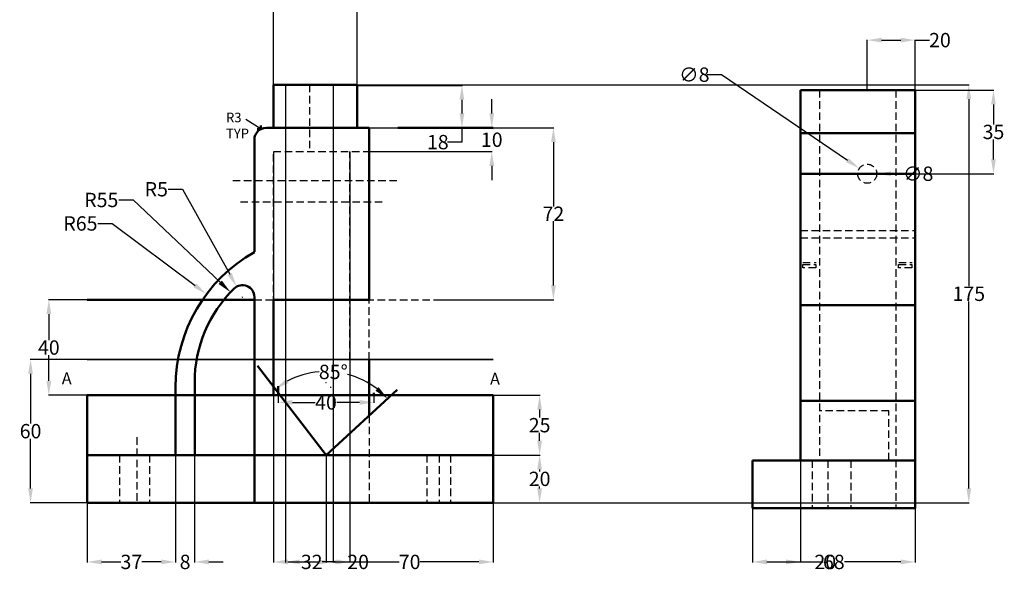
# Model space of a CAD drawing. Units: inches. Extents: x 537 to 975, y 162 to 623.
# Tile 1 of 2: x 563 to 975, y 162 to 393. Entities that reach past the tile are written whole.
import ezdxf

# ---------------------------------------------------------------- set-up
doc = ezdxf.new("R2010")
doc.units = ezdxf.units.IN
doc.header["$LTSCALE"] = 5
doc.header["$MEASUREMENT"] = 0
doc.linetypes.add('HIDDEN2', pattern=[0.1875, 0.125, -0.0625])
doc.linetypes.add('PHANTOM', pattern=[63.5, 31.75, -6.35, 6.35, -6.35, 6.35, -6.35])
for name, color, linetype, lineweight in [('M-DIMS', 2, 'Continuous', 25), ('M-HIDN', 4, 'HIDDEN2', 25), ('M-OUTL', 7, 'Continuous', 50), ('M-SECT', 1, 'PHANTOM', 35), ('M-TEXT', 3, 'Continuous', 25)]:
    doc.layers.add(name, color=color, linetype=linetype, lineweight=lineweight)
doc.styles.get("Standard").update_dxf_attribs({"font": 'arial.ttf'})
doc.dimstyles.get("Standard").update_dxf_attribs({"dimtxt": 6, "dimasz": 6, "dimexe": 0.18, "dimexo": 0.0625, "dimgap": 0.09, "dimtad": 0, "dimtih": 1, "dimtoh": 1, "dimdec": 0, "dimzin": 0, "dimdsep": 46, "dimtxsty": 'Standard', "dimcen": 0.09, "dimadec": 0, "dimazin": 0, "dimtfac": 1, "dimtdec": 0, "dimtofl": 0, "dimtmove": 0, "dimatfit": 3, "dimfxl": 1, "dimtolj": 1, "dimtzin": 0, "dimarcsym": 0})

# ---------------------------------------------------------------- blocks, each defined once
blk = doc.blocks.new('*D15')
at = {"layer": 'Defpoints', "color": 0, "lineweight": 30, "ltscale": 5, "transparency": 16777216}
for p in [(662.25, 248.32), (702.39, 243.97), (720.66, 238.22), (690.92, 210.97), (690.92, 210.97)]:
    blk.add_point(p, dxfattribs=at)
at = {"layer": 'M-DIMS', "color": 0, "lineweight": -2, "ltscale": 5, "transparency": 16777216}
for start, end in [(94.8184, 117.6478), (52.3522, 75.0302)]:
    blk.add_arc((690.92, 210.97), 34.94, start, end, dxfattribs=at)
at = {"layer": 'M-DIMS', "color": 0, "lineweight": 30, "ltscale": 5, "transparency": 16777216}
for points in [[(675.24, 241.07), (674.17, 242.76), (669.65, 238.68)], [(712.93, 239.37), (711.58, 237.89), (716.67, 234.57)]]:
    blk.add_solid(points, dxfattribs=at)
at = {"layer": 'M-DIMS', "color": 0, "ltscale": 5, "transparency": 16777216, "insert": (693.96, 245.77), "char_height": 6, "attachment_point": 5}
blk.add_mtext('\\A1;85°', dxfattribs=at)
blk = doc.blocks.new('*D16')
at = {"layer": 'Defpoints', "color": 0, "lineweight": 30, "ltscale": 5, "transparency": 16777216}
for p in [(670.86, 235.97), (710.92, 235.97), (710.92, 233.01)]:
    blk.add_point(p, dxfattribs=at)
at = {"layer": 'M-DIMS', "color": 0, "lineweight": -2, "ltscale": 5, "transparency": 16777216}
for p, q in [((670.86, 235.9), (670.86, 232.83)), ((710.92, 235.9), (710.92, 232.83)), ((676.86, 233.01), (686.39, 233.01)), ((704.92, 233.01), (695.38, 233.01))]:
    blk.add_line(p, q, dxfattribs=at)
at = {"layer": 'M-DIMS', "color": 0, "lineweight": 30, "ltscale": 5, "transparency": 16777216}
for points in [[(676.86, 234.01), (676.86, 232.01), (670.86, 233.01)], [(704.92, 234.01), (704.92, 232.01), (710.92, 233.01)]]:
    blk.add_solid(points, dxfattribs=at)
at = {"layer": 'M-DIMS', "color": 0, "ltscale": 5, "transparency": 16777216, "insert": (690.89, 233.01), "char_height": 6, "attachment_point": 5}
blk.add_mtext('\\A1;40', dxfattribs=at)
blk = doc.blocks.new('*D17')
at = {"layer": 'Defpoints', "color": 0, "lineweight": 30, "ltscale": 5, "transparency": 16777216}
for p in [(760.92, 210.97), (780.32, 210.97), (758.37, 191.01)]:
    blk.add_point(p, dxfattribs=at)
at = {"layer": 'M-DIMS', "color": 0, "lineweight": -2, "ltscale": 5, "transparency": 16777216}
for p, q in [((760.98, 210.97), (780.5, 210.97)), ((780.32, 204.97), (780.32, 204.14)), ((780.32, 197.01), (780.32, 197.84)), ((758.44, 191.01), (780.5, 191.01))]:
    blk.add_line(p, q, dxfattribs=at)
at = {"layer": 'M-DIMS', "color": 0, "lineweight": 30, "ltscale": 5, "transparency": 16777216}
for points in [[(779.32, 204.97), (781.32, 204.97), (780.32, 210.97)], [(779.32, 197.01), (781.32, 197.01), (780.32, 191.01)]]:
    blk.add_solid(points, dxfattribs=at)
at = {"layer": 'M-DIMS', "color": 0, "ltscale": 5, "transparency": 16777216, "insert": (780.32, 200.99), "char_height": 6, "attachment_point": 5}
blk.add_mtext('\\A1;20', dxfattribs=at)
blk = doc.blocks.new('*D18')
at = {"layer": 'Defpoints', "color": 0, "lineweight": 30, "ltscale": 5, "transparency": 16777216}
for p in [(760.92, 235.97), (780.32, 235.97), (760.92, 210.97)]:
    blk.add_point(p, dxfattribs=at)
at = {"layer": 'M-DIMS', "color": 0, "lineweight": -2, "ltscale": 5, "transparency": 16777216}
for p, q in [((760.98, 235.97), (780.5, 235.97)), ((780.32, 229.97), (780.32, 226.62)), ((780.32, 216.97), (780.32, 220.31)), ((760.98, 210.97), (780.5, 210.97))]:
    blk.add_line(p, q, dxfattribs=at)
at = {"layer": 'M-DIMS', "color": 0, "lineweight": 30, "ltscale": 5, "transparency": 16777216}
for points in [[(779.32, 229.97), (781.32, 229.97), (780.32, 235.97)], [(779.32, 216.97), (781.32, 216.97), (780.32, 210.97)]]:
    blk.add_solid(points, dxfattribs=at)
at = {"layer": 'M-DIMS', "color": 0, "ltscale": 5, "transparency": 16777216, "insert": (780.32, 223.47), "char_height": 6, "attachment_point": 5}
blk.add_mtext('\\A1;25', dxfattribs=at)
blk = doc.blocks.new('*D19')
at = {"layer": 'Defpoints', "color": 0, "lineweight": 30, "ltscale": 5, "transparency": 16777216}
for p in [(567.22, 250.97), (590.92, 250.97), (590.92, 190.97)]:
    blk.add_point(p, dxfattribs=at)
at = {"layer": 'M-DIMS', "color": 0, "lineweight": -2, "ltscale": 5, "transparency": 16777216}
for p, q in [((590.85, 250.97), (567.04, 250.97)), ((567.22, 244.97), (567.22, 224.12)), ((567.22, 196.97), (567.22, 217.81)), ((590.85, 190.97), (567.04, 190.97))]:
    blk.add_line(p, q, dxfattribs=at)
at = {"layer": 'M-DIMS', "color": 0, "lineweight": 30, "ltscale": 5, "transparency": 16777216}
for points in [[(566.22, 244.97), (568.22, 244.97), (567.22, 250.97)], [(566.22, 196.97), (568.22, 196.97), (567.22, 190.97)]]:
    blk.add_solid(points, dxfattribs=at)
at = {"layer": 'M-DIMS', "color": 0, "ltscale": 5, "transparency": 16777216, "insert": (567.22, 220.97), "char_height": 6, "attachment_point": 5}
blk.add_mtext('\\A1;60', dxfattribs=at)
blk = doc.blocks.new('*D20')
at = {"layer": 'Defpoints', "color": 0, "lineweight": 30, "ltscale": 5, "transparency": 16777216}
for p in [(574.87, 275.97), (590.92, 275.97), (590.92, 235.97)]:
    blk.add_point(p, dxfattribs=at)
at = {"layer": 'M-DIMS', "color": 0, "lineweight": -2, "ltscale": 5, "transparency": 16777216}
for p, q in [((590.85, 275.97), (574.69, 275.97)), ((574.87, 269.97), (574.87, 259.12)), ((574.87, 241.97), (574.87, 252.81)), ((590.85, 235.97), (574.69, 235.97))]:
    blk.add_line(p, q, dxfattribs=at)
at = {"layer": 'M-DIMS', "color": 0, "lineweight": 30, "ltscale": 5, "transparency": 16777216}
for points in [[(573.87, 269.97), (575.87, 269.97), (574.87, 275.97)], [(573.87, 241.97), (575.87, 241.97), (574.87, 235.97)]]:
    blk.add_solid(points, dxfattribs=at)
at = {"layer": 'M-DIMS', "color": 0, "ltscale": 5, "transparency": 16777216, "insert": (574.87, 255.97), "char_height": 6, "attachment_point": 5}
blk.add_mtext('\\A1;40', dxfattribs=at)
blk = doc.blocks.new('*D21')
at = {"layer": 'Defpoints', "color": 0, "lineweight": 30, "ltscale": 5, "transparency": 16777216}
for p in [(737.44, 347.97), (786.09, 347.97), (737.44, 275.97)]:
    blk.add_point(p, dxfattribs=at)
at = {"layer": 'M-DIMS', "color": 0, "lineweight": -2, "ltscale": 5, "transparency": 16777216}
for p, q in [((737.5, 347.97), (786.27, 347.97)), ((786.09, 341.97), (786.09, 315.07)), ((786.09, 281.97), (786.09, 308.87)), ((737.5, 275.97), (786.27, 275.97))]:
    blk.add_line(p, q, dxfattribs=at)
at = {"layer": 'M-DIMS', "color": 0, "lineweight": 30, "ltscale": 5, "transparency": 16777216}
for points in [[(785.09, 341.97), (787.09, 341.97), (786.09, 347.97)], [(785.09, 281.97), (787.09, 281.97), (786.09, 275.97)]]:
    blk.add_solid(points, dxfattribs=at)
at = {"layer": 'M-DIMS', "color": 0, "ltscale": 5, "transparency": 16777216, "insert": (786.09, 311.97), "char_height": 6, "attachment_point": 5}
blk.add_mtext('\\A1;72', dxfattribs=at)
blk = doc.blocks.new('*D22')
at = {"layer": 'Defpoints', "color": 0, "lineweight": 30, "ltscale": 5, "transparency": 16777216}
for p in [(708.92, 347.97), (760.28, 347.97), (708.92, 337.97)]:
    blk.add_point(p, dxfattribs=at)
at = {"layer": 'M-DIMS', "color": 0, "lineweight": -2, "ltscale": 5, "transparency": 16777216}
for p, q in [((760.28, 353.97), (760.28, 359.97)), ((708.98, 347.97), (760.46, 347.97)), ((708.98, 337.97), (760.46, 337.97)), ((760.28, 331.97), (760.28, 325.97))]:
    blk.add_line(p, q, dxfattribs=at)
at = {"layer": 'M-DIMS', "color": 0, "lineweight": 30, "ltscale": 5, "transparency": 16777216}
for points in [[(759.28, 353.97), (761.28, 353.97), (760.28, 347.97)], [(759.28, 331.97), (761.28, 331.97), (760.28, 337.97)]]:
    blk.add_solid(points, dxfattribs=at)
at = {"layer": 'M-DIMS', "color": 0, "ltscale": 5, "transparency": 16777216, "insert": (760.28, 342.97), "char_height": 6, "attachment_point": 5}
blk.add_mtext('\\A1;10', dxfattribs=at)
blk = doc.blocks.new('*D23')
at = {"layer": 'Defpoints', "color": 0, "lineweight": 30, "ltscale": 5, "transparency": 16777216}
for p in [(703.92, 365.68), (703.92, 347.97), (747.8, 347.97)]:
    blk.add_point(p, dxfattribs=at)
at = {"layer": 'M-DIMS', "color": 0, "lineweight": -2, "ltscale": 5, "transparency": 16777216}
for p, q in [((703.98, 365.68), (747.98, 365.68)), ((747.8, 359.68), (747.8, 353.97)), ((703.98, 347.97), (747.98, 347.97)), ((747.8, 347.97), (747.8, 341.97)), ((747.8, 341.97), (741.8, 341.97))]:
    blk.add_line(p, q, dxfattribs=at)
at = {"layer": 'M-DIMS', "color": 0, "lineweight": 30, "ltscale": 5, "transparency": 16777216}
for points in [[(746.8, 359.68), (748.8, 359.68), (747.8, 365.68)], [(746.8, 353.97), (748.8, 353.97), (747.8, 347.97)]]:
    blk.add_solid(points, dxfattribs=at)
at = {"layer": 'M-DIMS', "color": 0, "ltscale": 5, "transparency": 16777216, "insert": (737.69, 341.97), "char_height": 6, "attachment_point": 5}
blk.add_mtext('\\A1;18', dxfattribs=at)
blk = doc.blocks.new('*D24')
at = {"layer": 'Defpoints', "color": 0, "lineweight": 30, "ltscale": 5, "transparency": 16777216}
for p in [(653.49, 281.47), (655.92, 277.1)]:
    blk.add_point(p, dxfattribs=at)
at = {"layer": 'M-DIMS', "color": 0, "lineweight": -2, "ltscale": 5, "transparency": 16777216}
for p, q in [((624.82, 322.24), (630.82, 322.24)), ((630.82, 322.24), (650.57, 286.71)), ((655.83, 277.1), (656.01, 277.1)), ((655.92, 277.01), (655.92, 277.19))]:
    blk.add_line(p, q, dxfattribs=at)
at = {"layer": 'M-DIMS', "color": 0, "lineweight": 30, "ltscale": 5, "transparency": 16777216}
blk.add_solid([(651.44, 287.2), (649.7, 286.23), (653.49, 281.47)], dxfattribs=at)
at = {"layer": 'M-DIMS', "color": 0, "ltscale": 5, "transparency": 16777216, "insert": (619.86, 322.24), "char_height": 6, "attachment_point": 5}
blk.add_mtext('\\A1;R5', dxfattribs=at)
blk = doc.blocks.new('*D25')
at = {"layer": 'Defpoints', "color": 0, "lineweight": 30, "ltscale": 5, "transparency": 16777216}
for p in [(640.88, 278.34), (692.92, 239.39)]:
    blk.add_point(p, dxfattribs=at)
at = {"layer": 'M-DIMS', "color": 0, "lineweight": -2, "ltscale": 5, "transparency": 16777216}
for p, q in [((595.38, 307.91), (601.38, 307.91)), ((601.38, 307.91), (636.07, 281.94)), ((692.83, 239.39), (693.01, 239.39)), ((692.92, 239.3), (692.92, 239.48))]:
    blk.add_line(p, q, dxfattribs=at)
at = {"layer": 'M-DIMS', "color": 0, "lineweight": 30, "ltscale": 5, "transparency": 16777216}
blk.add_solid([(636.67, 282.74), (635.47, 281.14), (640.88, 278.34)], dxfattribs=at)
at = {"layer": 'M-DIMS', "color": 0, "ltscale": 5, "transparency": 16777216, "insert": (588.1, 307.91), "char_height": 6, "attachment_point": 5}
blk.add_mtext('\\A1;R65', dxfattribs=at)
blk = doc.blocks.new('*D26')
at = {"layer": 'Defpoints', "color": 0, "lineweight": 30, "ltscale": 5, "transparency": 16777216}
for p in [(650.94, 279.17), (690.92, 241.39)]:
    blk.add_point(p, dxfattribs=at)
at = {"layer": 'M-DIMS', "color": 0, "lineweight": -2, "ltscale": 5, "transparency": 16777216}
for p, q in [((604.11, 317.75), (610.11, 317.75)), ((610.11, 317.75), (646.58, 283.29)), ((690.83, 241.39), (691.01, 241.39)), ((690.92, 241.3), (690.92, 241.48))]:
    blk.add_line(p, q, dxfattribs=at)
at = {"layer": 'M-DIMS', "color": 0, "lineweight": 30, "ltscale": 5, "transparency": 16777216}
blk.add_solid([(647.27, 284.02), (645.89, 282.56), (650.94, 279.17)], dxfattribs=at)
at = {"layer": 'M-DIMS', "color": 0, "ltscale": 5, "transparency": 16777216, "insert": (596.83, 317.75), "char_height": 6, "attachment_point": 5}
blk.add_mtext('\\A1;R55', dxfattribs=at)
blk = doc.blocks.new('*D27')
at = {"layer": 'Defpoints', "color": 0, "lineweight": 30, "ltscale": 5, "transparency": 16777216}
for p in [(914.16, 330.98), (920.78, 326.49)]:
    blk.add_point(p, dxfattribs=at)
at = {"layer": 'M-DIMS', "color": 0, "lineweight": -2, "ltscale": 5, "transparency": 16777216}
for p, q in [((850.41, 370.21), (856.41, 370.21)), ((856.41, 370.21), (909.2, 334.35)), ((917.38, 328.73), (917.56, 328.73)), ((917.47, 328.64), (917.47, 328.82))]:
    blk.add_line(p, q, dxfattribs=at)
at = {"layer": 'M-DIMS', "color": 0, "lineweight": 30, "ltscale": 5, "transparency": 16777216}
blk.add_solid([(909.76, 335.18), (908.63, 333.53), (914.16, 330.98)], dxfattribs=at)
at = {"layer": 'M-DIMS', "color": 0, "ltscale": 5, "transparency": 16777216, "insert": (845.08, 370.21), "char_height": 6, "attachment_point": 5}
blk.add_mtext('\\A1;∅8', dxfattribs=at)
blk = doc.blocks.new('*D28')
at = {"layer": 'Defpoints', "color": 0, "lineweight": 30, "ltscale": 5, "transparency": 16777216}
for p in [(937.47, 384.67), (917.47, 363.73), (937.47, 363.73)]:
    blk.add_point(p, dxfattribs=at)
at = {"layer": 'M-DIMS', "color": 0, "lineweight": -2, "ltscale": 5, "transparency": 16777216}
for p, q in [((917.47, 363.8), (917.47, 384.85)), ((923.47, 384.67), (931.47, 384.67)), ((937.47, 363.8), (937.47, 384.85)), ((937.47, 384.67), (943.47, 384.67))]:
    blk.add_line(p, q, dxfattribs=at)
at = {"layer": 'M-DIMS', "color": 0, "lineweight": 30, "ltscale": 5, "transparency": 16777216}
for points in [[(923.47, 385.67), (923.47, 383.67), (917.47, 384.67)], [(931.47, 385.67), (931.47, 383.67), (937.47, 384.67)]]:
    blk.add_solid(points, dxfattribs=at)
at = {"layer": 'M-DIMS', "color": 0, "ltscale": 5, "transparency": 16777216, "insert": (947.9, 384.67), "char_height": 6, "attachment_point": 5}
blk.add_mtext('\\A1;20', dxfattribs=at)
blk = doc.blocks.new('*D29')
at = {"layer": 'Defpoints', "color": 0, "lineweight": 30, "ltscale": 5, "transparency": 16777216}
for p in [(937.47, 363.73), (937.47, 328.73), (970.3, 328.73)]:
    blk.add_point(p, dxfattribs=at)
at = {"layer": 'M-DIMS', "color": 0, "lineweight": -2, "ltscale": 5, "transparency": 16777216}
for p, q in [((937.53, 363.73), (970.48, 363.73)), ((970.3, 357.73), (970.3, 349.39)), ((970.3, 334.73), (970.3, 343.08)), ((937.53, 328.73), (970.48, 328.73))]:
    blk.add_line(p, q, dxfattribs=at)
at = {"layer": 'M-DIMS', "color": 0, "lineweight": 30, "ltscale": 5, "transparency": 16777216}
for points in [[(969.3, 357.73), (971.3, 357.73), (970.3, 363.73)], [(969.3, 334.73), (971.3, 334.73), (970.3, 328.73)]]:
    blk.add_solid(points, dxfattribs=at)
at = {"layer": 'M-DIMS', "color": 0, "ltscale": 5, "transparency": 16777216, "insert": (970.3, 346.23), "char_height": 6, "attachment_point": 5}
blk.add_mtext('\\A1;35', dxfattribs=at)
blk = doc.blocks.new('*D30')
at = {"layer": 'Defpoints', "color": 0, "lineweight": 30, "ltscale": 5, "transparency": 16777216}
for p in [(627.92, 239.39), (590.92, 190.97), (627.92, 166.23)]:
    blk.add_point(p, dxfattribs=at)
at = {"layer": 'M-DIMS', "color": 0, "lineweight": -2, "ltscale": 5, "transparency": 16777216}
for p, q in [((627.92, 239.33), (627.92, 166.05)), ((590.92, 190.9), (590.92, 166.05)), ((596.92, 166.23), (605.03, 166.23)), ((621.92, 166.23), (613.8, 166.23))]:
    blk.add_line(p, q, dxfattribs=at)
at = {"layer": 'M-DIMS', "color": 0, "lineweight": 30, "ltscale": 5, "transparency": 16777216}
for points in [[(596.92, 167.23), (596.92, 165.23), (590.92, 166.23)], [(621.92, 167.23), (621.92, 165.23), (627.92, 166.23)]]:
    blk.add_solid(points, dxfattribs=at)
at = {"layer": 'M-DIMS', "color": 0, "ltscale": 5, "transparency": 16777216, "insert": (609.42, 166.23), "char_height": 6, "attachment_point": 5}
blk.add_mtext('\\A1;37', dxfattribs=at)
blk = doc.blocks.new('*D31')
at = {"layer": 'Defpoints', "color": 0, "lineweight": 30, "ltscale": 5, "transparency": 16777216}
for p in [(627.91595, 210.967485), (635.91595, 210.967485), (635.91595, 166.233266)]:
    blk.add_point(p, dxfattribs=at)
at = {"layer": 'M-DIMS', "color": 0, "lineweight": -2, "ltscale": 5, "transparency": 16777216}
for p, q in [((627.91595, 210.904985), (627.91595, 166.053266)), ((635.91595, 210.904985), (635.91595, 166.053266)), ((621.91595, 166.233266), (615.91595, 166.233266)), ((641.91595, 166.233266), (647.91595, 166.233266))]:
    blk.add_line(p, q, dxfattribs=at)
at = {"layer": 'M-DIMS', "color": 0, "lineweight": 30, "ltscale": 5, "transparency": 16777216}
for points in [[(621.91595, 167.233266), (621.91595, 165.233266), (627.91595, 166.233266)], [(641.91595, 167.233266), (641.91595, 165.233266), (635.91595, 166.233266)]]:
    blk.add_solid(points, dxfattribs=at)
at = {"layer": 'M-DIMS', "color": 0, "ltscale": 5, "transparency": 16777216, "insert": (631.91595, 166.233266), "char_height": 6, "attachment_point": 5}
blk.add_mtext('\\A1;8', dxfattribs=at)
blk = doc.blocks.new('*D32')
at = {"layer": 'Defpoints', "color": 0, "lineweight": 30, "ltscale": 5, "transparency": 16777216}
for p in [(690.92, 210.97), (760.92, 190.97), (690.92, 166.23)]:
    blk.add_point(p, dxfattribs=at)
at = {"layer": 'M-DIMS', "color": 0, "lineweight": -2, "ltscale": 5, "transparency": 16777216}
for p, q in [((690.92, 210.9), (690.92, 166.05)), ((760.92, 190.9), (760.92, 166.05)), ((696.92, 166.23), (721.56, 166.23)), ((754.92, 166.23), (730.27, 166.23))]:
    blk.add_line(p, q, dxfattribs=at)
at = {"layer": 'M-DIMS', "color": 0, "lineweight": 30, "ltscale": 5, "transparency": 16777216}
for points in [[(696.92, 167.23), (696.92, 165.23), (690.92, 166.23)], [(754.92, 167.23), (754.92, 165.23), (760.92, 166.23)]]:
    blk.add_solid(points, dxfattribs=at)
at = {"layer": 'M-DIMS', "color": 0, "ltscale": 5, "transparency": 16777216, "insert": (725.92, 166.23), "char_height": 6, "attachment_point": 5}
blk.add_mtext('\\A1;70', dxfattribs=at)
blk = doc.blocks.new('*D33')
at = {"layer": 'Defpoints', "color": 0, "lineweight": 30, "ltscale": 5, "transparency": 16777216}
for p in [(703.92, 619.5), (668.92, 365.97), (703.92, 365.97)]:
    blk.add_point(p, dxfattribs=at)
at = {"layer": 'M-DIMS', "color": 0, "lineweight": -2, "ltscale": 5, "transparency": 16777216}
for p, q in [((668.92, 366.03), (668.92, 619.68)), ((674.92, 619.5), (682.01, 619.5)), ((697.92, 619.5), (690.82, 619.5)), ((703.92, 366.03), (703.92, 619.68))]:
    blk.add_line(p, q, dxfattribs=at)
at = {"layer": 'M-DIMS', "color": 0, "lineweight": 30, "ltscale": 5, "transparency": 16777216}
for points in [[(674.92, 620.5), (674.92, 618.5), (668.92, 619.5)], [(697.92, 620.5), (697.92, 618.5), (703.92, 619.5)]]:
    blk.add_solid(points, dxfattribs=at)
at = {"layer": 'M-DIMS', "color": 0, "ltscale": 5, "transparency": 16777216, "insert": (686.42, 619.5), "char_height": 6, "attachment_point": 5}
blk.add_mtext('\\A1;35', dxfattribs=at)
blk = doc.blocks.new('*D34')
at = {"layer": 'Defpoints', "color": 0, "lineweight": 30, "ltscale": 5, "transparency": 16777216}
for p in [(668.92, 337.97), (700.92, 337.97), (700.92, 166.23)]:
    blk.add_point(p, dxfattribs=at)
at = {"layer": 'M-DIMS', "color": 0, "lineweight": -2, "ltscale": 5, "transparency": 16777216}
for p, q in [((668.92, 337.9), (668.92, 166.05)), ((700.92, 337.9), (700.92, 166.05)), ((674.92, 166.23), (680.56, 166.23)), ((694.92, 166.23), (689.27, 166.23))]:
    blk.add_line(p, q, dxfattribs=at)
at = {"layer": 'M-DIMS', "color": 0, "lineweight": 30, "ltscale": 5, "transparency": 16777216}
for points in [[(674.92, 167.23), (674.92, 165.23), (668.92, 166.23)], [(694.92, 167.23), (694.92, 165.23), (700.92, 166.23)]]:
    blk.add_solid(points, dxfattribs=at)
at = {"layer": 'M-DIMS', "color": 0, "ltscale": 5, "transparency": 16777216, "insert": (684.92, 166.23), "char_height": 6, "attachment_point": 5}
blk.add_mtext('\\A1;32', dxfattribs=at)
blk = doc.blocks.new('*D35')
at = {"layer": 'Defpoints', "color": 0, "lineweight": 30, "ltscale": 5, "transparency": 16777216}
for p in [(673.92, 365.97), (693.92, 365.97), (693.92, 166.23)]:
    blk.add_point(p, dxfattribs=at)
at = {"layer": 'M-DIMS', "color": 0, "lineweight": -2, "ltscale": 5, "transparency": 16777216}
for p, q in [((673.92, 365.9), (673.92, 166.05)), ((693.92, 365.9), (693.92, 166.05)), ((679.92, 166.23), (687.92, 166.23)), ((693.92, 166.23), (699.92, 166.23))]:
    blk.add_line(p, q, dxfattribs=at)
at = {"layer": 'M-DIMS', "color": 0, "lineweight": 30, "ltscale": 5, "transparency": 16777216}
for points in [[(679.92, 167.23), (679.92, 165.23), (673.92, 166.23)], [(687.92, 167.23), (687.92, 165.23), (693.92, 166.23)]]:
    blk.add_solid(points, dxfattribs=at)
at = {"layer": 'M-DIMS', "color": 0, "ltscale": 5, "transparency": 16777216, "insert": (704.34, 166.23), "char_height": 6, "attachment_point": 5}
blk.add_mtext('\\A1;20', dxfattribs=at)
blk = doc.blocks.new('*D36')
at = {"layer": 'Defpoints', "color": 0, "lineweight": 30, "ltscale": 5, "transparency": 16777216}
for p in [(703.92, 365.97), (959.97, 365.97), (760.92, 190.97)]:
    blk.add_point(p, dxfattribs=at)
at = {"layer": 'M-DIMS', "color": 0, "lineweight": -2, "ltscale": 5, "transparency": 16777216}
for p, q in [((703.98, 365.97), (960.15, 365.97)), ((959.97, 359.97), (959.97, 281.62)), ((959.97, 196.97), (959.97, 275.31)), ((760.98, 190.97), (960.15, 190.97))]:
    blk.add_line(p, q, dxfattribs=at)
at = {"layer": 'M-DIMS', "color": 0, "lineweight": 30, "ltscale": 5, "transparency": 16777216}
for points in [[(958.97, 359.97), (960.97, 359.97), (959.97, 365.97)], [(958.97, 196.97), (960.97, 196.97), (959.97, 190.97)]]:
    blk.add_solid(points, dxfattribs=at)
at = {"layer": 'M-DIMS', "color": 0, "ltscale": 5, "transparency": 16777216, "insert": (959.97, 278.47), "char_height": 6, "attachment_point": 5}
blk.add_mtext('\\A1;175', dxfattribs=at)
blk = doc.blocks.new('*D37')
at = {"layer": 'Defpoints', "color": 0, "lineweight": 30, "ltscale": 5, "transparency": 16777216}
for p in [(869.47, 188.73), (937.47, 188.73), (937.47, 166.23)]:
    blk.add_point(p, dxfattribs=at)
at = {"layer": 'M-DIMS', "color": 0, "lineweight": -2, "ltscale": 5, "transparency": 16777216}
for p, q in [((869.47, 188.67), (869.47, 166.05)), ((937.47, 188.67), (937.47, 166.05)), ((875.47, 166.23), (899.06, 166.23)), ((931.47, 166.23), (907.88, 166.23))]:
    blk.add_line(p, q, dxfattribs=at)
at = {"layer": 'M-DIMS', "color": 0, "lineweight": 30, "ltscale": 5, "transparency": 16777216}
for points in [[(875.47, 167.23), (875.47, 165.23), (869.47, 166.23)], [(931.47, 167.23), (931.47, 165.23), (937.47, 166.23)]]:
    blk.add_solid(points, dxfattribs=at)
at = {"layer": 'M-DIMS', "color": 0, "ltscale": 5, "transparency": 16777216, "insert": (903.47, 166.23), "char_height": 6, "attachment_point": 5}
blk.add_mtext('\\A1;68', dxfattribs=at)
blk = doc.blocks.new('*D38')
at = {"layer": 'Defpoints', "color": 0, "lineweight": 30, "ltscale": 5, "transparency": 16777216}
for p in [(869.47, 208.73), (889.47, 208.73), (889.47, 166.23)]:
    blk.add_point(p, dxfattribs=at)
at = {"layer": 'M-DIMS', "color": 0, "lineweight": -2, "ltscale": 5, "transparency": 16777216}
for p, q in [((869.47, 208.67), (869.47, 166.05)), ((889.47, 208.67), (889.47, 166.05)), ((875.47, 166.23), (883.47, 166.23)), ((889.47, 166.23), (895.47, 166.23))]:
    blk.add_line(p, q, dxfattribs=at)
at = {"layer": 'M-DIMS', "color": 0, "lineweight": 30, "ltscale": 5, "transparency": 16777216}
for points in [[(875.47, 167.23), (875.47, 165.23), (869.47, 166.23)], [(883.47, 167.23), (883.47, 165.23), (889.47, 166.23)]]:
    blk.add_solid(points, dxfattribs=at)
at = {"layer": 'M-DIMS', "color": 0, "ltscale": 5, "transparency": 16777216, "insert": (899.9, 166.23), "char_height": 6, "attachment_point": 5}
blk.add_mtext('\\A1;20', dxfattribs=at)
blk = doc.blocks.new('*D41')
at = {"layer": 'Defpoints', "color": 0, "lineweight": 30, "ltscale": 5, "transparency": 16777216}
for p in [(913.47, 328.73), (921.47, 328.73)]:
    blk.add_point(p, dxfattribs=at)
at = {"layer": 'M-DIMS', "color": 0, "lineweight": -2, "ltscale": 5, "transparency": 16777216}
for p, q in [((917.38, 328.73), (917.56, 328.73)), ((917.47, 328.64), (917.47, 328.82)), ((933.47, 328.73), (927.47, 328.73))]:
    blk.add_line(p, q, dxfattribs=at)
at = {"layer": 'M-DIMS', "color": 0, "lineweight": 30, "ltscale": 5, "transparency": 16777216}
blk.add_solid([(927.47, 329.73), (927.47, 327.73), (921.47, 328.73)], dxfattribs=at)
at = {"layer": 'M-DIMS', "color": 0, "ltscale": 5, "transparency": 16777216, "insert": (938.79, 328.73), "char_height": 6, "attachment_point": 5}
blk.add_mtext('\\A1;∅8', dxfattribs=at)

msp = doc.modelspace()

# ---------------------------------------------------------------- linework, layer by layer
at = {"layer": 'M-DIMS', "ltscale": 5}
msp.add_line((663.71, 347.45), (657.28, 351.44), dxfattribs=at)
at = {"layer": 'M-HIDN', "ltscale": 5}
for p, q in [((668.92, 347.97), (668.92, 365.97)), ((673.92, 365.97), (673.92, 337.97)), ((683.92, 365.97), (683.92, 337.97)), ((693.92, 365.97), (693.92, 337.97)), ((703.92, 365.97), (703.92, 347.97)), ((897.47, 363.73), (897.47, 208.73)), ((929.47, 363.73), (929.47, 188.73)), ((660.92, 295.97), (660.92, 342.97)), ((668.92, 291.6), (668.92, 337.97)), ((668.92, 337.97), (708.92, 337.97)), ((700.92, 250.97), (700.92, 337.97)), ((708.92, 250.97), (708.92, 337.97)), ((651.86, 325.94), (721.6, 325.94)), ((655.1, 316.99), (714.93, 316.99)), ((889.47, 304.92), (937.47, 304.92)), ((889.47, 301.92), (937.47, 301.92)), ((668.92, 250.97), (668.92, 291.6)), ((890.51, 291.55), (896.06, 291.55)), ((930.66, 291.55), (936.21, 291.55)), ((660.92, 275.97), (783.9, 275.97)), ((700.92, 250.97), (700.92, 190.97)), ((668.92, 235.97), (668.92, 190.97)), ((708.92, 227.46), (708.92, 190.97)), ((926.51, 229.45), (897.47, 229.45)), ((926.51, 208.73), (926.51, 229.45)), ((611.66, 218.4), (611.66, 190.97)), ((604.4, 210.97), (604.4, 190.97)), ((617.04, 210.97), (617.04, 190.97)), ((733.17, 210.97), (733.17, 190.97)), ((738.3, 210.97), (738.3, 190.97)), ((742.99, 210.97), (742.99, 190.97)), ((894.41, 208.73), (894.41, 188.73)), ((901.02, 208.73), (901.02, 188.73)), ((910.53, 208.73), (910.53, 188.73))]:
    msp.add_line(p, q, dxfattribs=at)
for points in [[(890.45, 290.78), (896.01, 290.78), (896.01, 289.4), (890.45, 289.4)], [(930.6, 290.78), (936.15, 290.78), (936.15, 289.4), (930.6, 289.4)]]:
    msp.add_lwpolyline(points, close=True, dxfattribs=at)
msp.add_circle((917.47, 328.73), 4, dxfattribs=at)
at = {"layer": 'M-OUTL', "ltscale": 5}
for p, q in [((668.92, 365.97), (703.92, 365.97)), ((703.92, 365.97), (668.92, 365.97)), ((668.92, 347.97), (668.92, 365.97)), ((668.92, 365.97), (703.92, 365.97)), ((703.92, 365.97), (703.92, 347.97)), ((889.47, 363.73), (937.47, 363.73)), ((889.47, 363.73), (889.47, 208.73)), ((937.47, 363.73), (937.47, 188.73)), ((663.71, 347.45), (662.07, 347.37)), ((663.71, 347.45), (663.64, 348.88)), ((665.92, 347.97), (708.92, 347.97)), ((665.92, 347.97), (668.92, 347.97)), ((703.92, 347.97), (708.92, 347.97)), ((708.92, 347.97), (708.92, 275.97)), ((720.92, 347.97), (760.92, 347.97)), ((660.92, 295.97), (660.92, 342.97)), ((889.47, 345.73), (937.47, 345.73)), ((889.47, 328.73), (937.47, 328.73)), ((660.92, 277.1), (660.92, 190.97)), ((590.92, 275.97), (660.92, 275.97)), ((668.92, 235.97), (668.92, 275.97)), ((668.92, 275.97), (708.92, 275.97)), ((889.47, 273.73), (937.47, 273.73)), ((690.92, 210.97), (662.25, 248.32)), ((668.92, 250.97), (668.92, 235.97)), ((708.92, 250.97), (708.92, 227.46)), ((627.92, 239.39), (627.92, 210.97)), ((635.92, 241.39), (635.92, 210.97)), ((670.92, 235.97), (670.86, 239.77)), ((590.92, 235.97), (760.92, 235.97)), ((590.92, 190.97), (590.92, 235.97)), ((710.92, 235.97), (670.92, 235.97)), ((700.92, 235.97), (680.92, 235.97)), ((690.92, 210.97), (720.66, 238.22)), ((690.92, 235.97), (710.92, 235.97)), ((710.92, 235.97), (710.92, 237.03)), ((760.92, 190.97), (760.92, 235.97)), ((889.47, 233.73), (937.47, 233.73)), ((590.92, 210.97), (760.92, 210.97)), ((720.92, 210.97), (660.92, 210.97)), ((869.47, 208.73), (937.47, 208.73)), ((869.47, 208.73), (869.47, 188.73)), ((590.92, 190.97), (760.92, 190.97)), ((869.47, 188.73), (937.47, 188.73))]:
    msp.add_line(p, q, dxfattribs=at)
for centre, radius, start, end in [((665.92, 342.97), 5, 90, 180), ((692.92, 239.39), 65, 119.4924, 180), ((690.92, 241.39), 55, 134.427, 180), ((655.92, 277.1), 5, 0, 134.427)]:
    msp.add_arc(centre, radius, start, end, dxfattribs=at)
at = {"layer": 'M-SECT', "ltscale": 5}
msp.add_line((590.92, 250.97), (760.92, 250.97), dxfattribs=at)

# ---------------------------------------------------------------- texts
at = {"layer": 'M-TEXT', "ltscale": 5, "attachment_point": 1}
for s, insert, char_height in [('R3\\PTYP', (649.04, 354.28), 4), ('A', (580.28, 245.53), 5), ('A', (759.56, 245.4), 5)]:
    msp.add_mtext_dynamic_manual_height_columns(s, width=21.8462, gutter_width=1, heights=[0], dxfattribs=dict(at, insert=insert, char_height=char_height))

# ---------------------------------------------------------------- dimensions: what is measured, and where the dimension line sits
at = {"layer": 'M-DIMS', "ltscale": 5}
for base, p1, p2, override, picture, middle in [((703.92, 619.5), (668.92, 365.97), (703.92, 365.97), {"dimdec": 0, "dimlfac": 1, "dimrnd": 0, "dimzin": 0, "dimdsep": 46, "dimlunit": 2}, '*D33', (686.42, 619.5)), ((937.47, 384.67), (917.47, 363.73), (937.47, 363.73), {"dimclrd": 0, "dimclre": 0, "dimclrt": 0}, '*D28', (947.9, 384.67)), ((693.92, 166.23), (673.92, 365.97), (693.92, 365.97), {"dimdec": 0, "dimlfac": 1, "dimrnd": 0, "dimzin": 0, "dimdsep": 46, "dimlunit": 2}, '*D35', (704.34, 166.23)), ((700.92, 166.23), (668.92, 337.97), (700.92, 337.97), {"dimdec": 0, "dimlfac": 1, "dimrnd": 0, "dimzin": 0, "dimdsep": 46, "dimlunit": 2}, '*D34', (684.92, 166.23)), ((627.92, 166.23), (590.92, 190.97), (627.92, 239.39), {"dimdec": 0, "dimlfac": 1, "dimrnd": 0, "dimzin": 0, "dimdsep": 46, "dimlunit": 2}, '*D30', (609.42, 166.23)), ((710.92, 233.01), (670.86, 235.97), (710.92, 235.97), {"dimclrd": 0, "dimclre": 0, "dimclrt": 0}, '*D16', (690.89, 233.01)), ((635.92, 166.23), (627.92, 210.97), (635.92, 210.97), {"dimdec": 0, "dimlfac": 1, "dimrnd": 0, "dimzin": 0, "dimdsep": 46, "dimlunit": 2}, '*D31', (631.92, 166.23)), ((690.92, 166.23), (760.92, 190.97), (690.92, 210.97), {"dimdec": 0, "dimlfac": 1, "dimrnd": 0, "dimzin": 0, "dimdsep": 46, "dimlunit": 2}, '*D32', (725.92, 166.23)), ((889.47, 166.23), (869.47, 208.73), (889.47, 208.73), {"dimdec": 0, "dimlfac": 1, "dimrnd": 0, "dimzin": 0, "dimdsep": 46, "dimlunit": 2}, '*D38', (899.9, 166.23)), ((937.47, 166.23), (869.47, 188.73), (937.47, 188.73), {"dimdec": 0, "dimlfac": 1, "dimrnd": 0, "dimzin": 0, "dimdsep": 46, "dimlunit": 2}, '*D37', (903.47, 166.23))]:
    dim = msp.add_linear_dim(base=base, p1=p1, p2=p2, dimstyle='Standard', override=override, dxfattribs=at)
    dim.commit()
    dim.dimension.update_dxf_attribs({"geometry": picture, "text_midpoint": middle})
for p1, p2, override, picture, middle in [((920.78, 326.49), (914.16, 330.98), {"dimclrd": 0, "dimclre": 0, "dimclrt": 0}, '*D27', (845.08, 370.21)), ((913.47, 328.73), (921.47, 328.73), {"dimdec": 0, "dimlfac": 1, "dimrnd": 0, "dimzin": 0, "dimdsep": 46, "dimlunit": 2}, '*D41', (933.47, 328.73))]:
    dim = msp.add_diameter_dim_2p(p1=p1, p2=p2, dimstyle='Standard', override=override, dxfattribs=at)
    dim.commit()
    dim.dimension.update_dxf_attribs({"geometry": picture, "text_midpoint": middle, "dimtype": 163})
for base, p1, p2, override, picture, middle in [((959.97, 365.97), (760.92, 190.97), (703.92, 365.97), {"dimdec": 0, "dimlfac": 1, "dimrnd": 0, "dimzin": 0, "dimdsep": 46, "dimlunit": 2}, '*D36', (959.97, 278.47)), ((747.8, 347.97), (703.92, 365.68), (703.92, 347.97), {"dimclrd": 0, "dimclre": 0, "dimclrt": 0}, '*D23', (737.69, 341.97)), ((970.3, 328.73), (937.47, 363.73), (937.47, 328.73), {"dimclrd": 0, "dimclre": 0, "dimclrt": 0}, '*D29', (970.3, 346.23)), ((760.28, 347.97), (708.92, 337.97), (708.92, 347.97), {"dimclrd": 0, "dimclre": 0, "dimclrt": 0}, '*D22', (760.28, 342.97)), ((786.09, 347.97), (737.44, 275.97), (737.44, 347.97), {"dimclrd": 0, "dimclre": 0, "dimclrt": 0}, '*D21', (786.09, 311.97)), ((574.87, 275.97), (590.92, 235.97), (590.92, 275.97), {"dimclrd": 0, "dimclre": 0, "dimclrt": 0}, '*D20', (574.87, 255.97)), ((567.22, 250.97), (590.92, 190.97), (590.92, 250.97), {"dimclrd": 0, "dimclre": 0, "dimclrt": 0}, '*D19', (567.22, 220.97)), ((780.32, 235.97), (760.92, 210.97), (760.92, 235.97), {"dimclrd": 0, "dimclre": 0, "dimclrt": 0}, '*D18', (780.32, 223.47)), ((780.32, 210.97), (758.37, 191.01), (760.92, 210.97), {"dimclrd": 0, "dimclre": 0, "dimclrt": 0}, '*D17', (780.32, 200.99))]:
    dim = msp.add_linear_dim(base=base, p1=p1, p2=p2, angle=90, dimstyle='Standard', override=override, dxfattribs=at)
    dim.commit()
    dim.dimension.update_dxf_attribs({"geometry": picture, "text_midpoint": middle})
for center, mpoint, picture, middle in [((655.92, 277.1), (653.49, 281.47), '*D24', (619.86, 322.24)), ((690.92, 241.39), (650.94, 279.17), '*D26', (596.83, 317.75)), ((692.92, 239.39), (640.88, 278.34), '*D25', (588.1, 307.91))]:
    dim = msp.add_radius_dim(center=center, mpoint=mpoint, dimstyle='Standard', override={"dimclrd": 0, "dimclre": 0, "dimclrt": 0}, dxfattribs=at)
    dim.commit()
    dim.dimension.update_dxf_attribs({"geometry": picture, "text_midpoint": middle, "dimtype": 164})
dim = msp.add_angular_dim_2l(base=(702.39, 243.97), line1=((690.92, 210.97), (720.66, 238.22)), line2=((690.92, 210.97), (662.25, 248.32)), dimstyle='Standard', override={"dimclrd": 0, "dimclre": 0, "dimclrt": 0}, dxfattribs=at)
dim.commit()
dim.dimension.update_dxf_attribs({"geometry": '*D15', "text_midpoint": (693.96, 245.77)})

doc.saveas('drawing.dxf')
